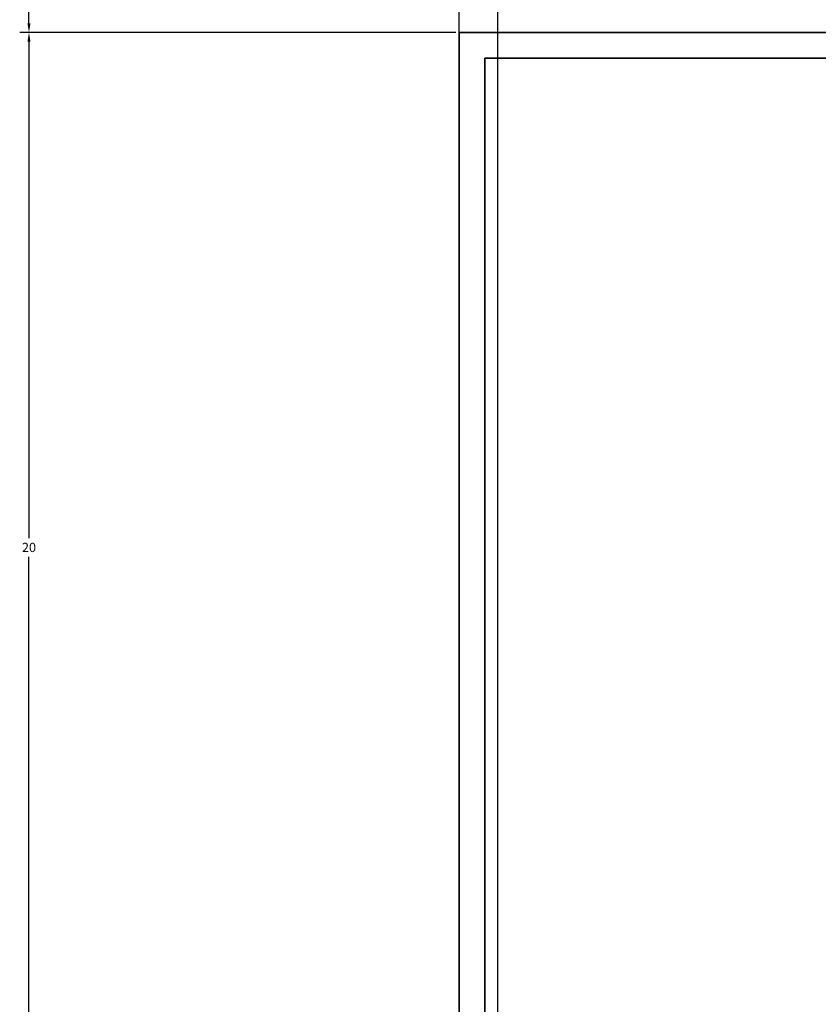
# Model space of a CAD drawing. Units: millimetres. Extents: x 446512 to 447461, y 70395 to 70610.
# Tile 2 of 39: x 446678.04 to 446693.54, y 70434.51 to 70453.63. Entities that reach past the tile are written whole.
import ezdxf

# ---------------------------------------------------------------- set-up
doc = ezdxf.new("R2010")
doc.units = ezdxf.units.MM
for name, color, linetype, lineweight in [('A-ANNO-DIMS', 2, 'Continuous', 18), ('A-CONS', 9, 'Continuous', 13), ('A-FURN', 7, 'Continuous', 35)]:
    doc.layers.add(name, color=color, linetype=linetype, lineweight=lineweight)
doc.styles.get("Standard").update_dxf_attribs({"font": 'arial.ttf'})
doc.dimstyles.get("Standard").update_dxf_attribs({"dimtxt": 0.18, "dimasz": 0.18, "dimexe": 0.18, "dimexo": 0.0625, "dimgap": 0.09, "dimtad": 0, "dimtih": 1, "dimtoh": 1, "dimdec": 4, "dimzin": 0, "dimdsep": 46, "dimtxsty": 'Standard', "dimcen": 0.09, "dimadec": 0, "dimazin": 0, "dimtfac": 1, "dimtdec": 4, "dimtofl": 0, "dimtmove": 0, "dimatfit": 3, "dimfxl": 1, "dimtolj": 1, "dimtzin": 0, "dimarcsym": 0})

# ---------------------------------------------------------------- blocks, each defined once
blk = doc.blocks.new('*D19')
at = {"layer": 'A-ANNO-DIMS', "color": 0, "lineweight": -2, "transparency": 16777216}
for p, q in [((446686.51, 70453.382), (446678.043, 70453.382)), ((446678.223, 70453.202), (446678.223, 70443.563)), ((446678.223, 70433.562), (446678.223, 70443.2)), ((446686.51, 70433.382), (446678.043, 70433.382))]:
    blk.add_line(p, q, dxfattribs=at)
at = {"layer": 'A-ANNO-DIMS', "color": 0, "transparency": 16777216}
for points in [[(446678.193, 70453.202), (446678.253, 70453.202), (446678.223, 70453.382)], [(446678.193, 70433.562), (446678.253, 70433.562), (446678.223, 70433.382)]]:
    blk.add_solid(points, dxfattribs=at)
at = {"layer": 'Defpoints', "color": 0, "transparency": 16777216}
for p in [(446678.223, 70453.382), (446686.573, 70453.382), (446686.573, 70433.382)]:
    blk.add_point(p, dxfattribs=at)
at = {"layer": 'A-ANNO-DIMS', "color": 0, "transparency": 16777216, "insert": (446678.223, 70443.382), "char_height": 0.18, "attachment_point": 5}
blk.add_mtext('\\A1;20', dxfattribs=at)
blk = doc.blocks.new('*D20')
at = {"layer": 'A-ANNO-DIMS', "color": 0, "lineweight": -2, "transparency": 16777216}
for p, q in [((446686.51, 70473.382), (446678.043, 70473.382)), ((446678.223, 70473.202), (446678.223, 70463.563)), ((446678.223, 70453.562), (446678.223, 70463.2)), ((446686.51, 70453.382), (446678.043, 70453.382))]:
    blk.add_line(p, q, dxfattribs=at)
at = {"layer": 'A-ANNO-DIMS', "color": 0, "transparency": 16777216}
for points in [[(446678.193, 70473.202), (446678.253, 70473.202), (446678.223, 70473.382)], [(446678.193, 70453.562), (446678.253, 70453.562), (446678.223, 70453.382)]]:
    blk.add_solid(points, dxfattribs=at)
at = {"layer": 'Defpoints', "color": 0, "transparency": 16777216}
for p in [(446678.223, 70473.382), (446686.573, 70473.382), (446686.573, 70453.382)]:
    blk.add_point(p, dxfattribs=at)
at = {"layer": 'A-ANNO-DIMS', "color": 0, "transparency": 16777216, "insert": (446678.223, 70463.382), "char_height": 0.18, "attachment_point": 5}
blk.add_mtext('\\A1;20', dxfattribs=at)
blk = doc.blocks.new('*D37')
at = {"layer": 'A-ANNO-DIMS', "color": 0, "lineweight": -2, "transparency": 16777216}
for p, q in [((446686.572846, 70433.44405), (446686.572846, 70578.17492)), ((446687.323552, 70428.838404), (446687.323552, 70578.17492)), ((446686.392846, 70577.99492), (446686.212846, 70577.99492)), ((446687.503552, 70577.99492), (446687.683552, 70577.99492))]:
    blk.add_line(p, q, dxfattribs=at)
at = {"layer": 'A-ANNO-DIMS', "color": 0, "transparency": 16777216}
for points in [[(446686.392846, 70578.02492), (446686.392846, 70577.96492), (446686.572846, 70577.99492)], [(446687.503552, 70578.02492), (446687.503552, 70577.96492), (446687.323552, 70577.99492)]]:
    blk.add_solid(points, dxfattribs=at)
at = {"layer": 'Defpoints', "color": 0, "transparency": 16777216}
for p in [(446687.323552, 70577.99492), (446686.572846, 70433.38155), (446687.323552, 70428.775904)]:
    blk.add_point(p, dxfattribs=at)
at = {"layer": 'A-ANNO-DIMS', "color": 0, "transparency": 16777216, "insert": (446686.948199, 70577.99492), "char_height": 0.18, "attachment_point": 5}
blk.add_mtext('\\A1;0.75', dxfattribs=at)
blk = doc.blocks.new('*D38')
at = {"layer": 'A-ANNO-DIMS', "color": 0, "lineweight": -2, "transparency": 16777216}
for p, q in [((446687.323552, 70428.838404), (446687.323552, 70578.17492)), ((446697.765686, 70428.838404), (446697.765686, 70578.17492)), ((446687.503552, 70577.99492), (446692.090383, 70577.99492)), ((446697.585686, 70577.99492), (446692.998855, 70577.99492))]:
    blk.add_line(p, q, dxfattribs=at)
at = {"layer": 'A-ANNO-DIMS', "color": 0, "transparency": 16777216}
for points in [[(446687.503552, 70578.02492), (446687.503552, 70577.96492), (446687.323552, 70577.99492)], [(446697.585686, 70578.02492), (446697.585686, 70577.96492), (446697.765686, 70577.99492)]]:
    blk.add_solid(points, dxfattribs=at)
at = {"layer": 'Defpoints', "color": 0, "transparency": 16777216}
for p in [(446697.765686, 70577.99492), (446687.323552, 70428.775904), (446697.765686, 70428.775904)]:
    blk.add_point(p, dxfattribs=at)
at = {"layer": 'A-ANNO-DIMS', "color": 0, "transparency": 16777216, "insert": (446692.544619, 70577.99492), "char_height": 0.18, "attachment_point": 5}
blk.add_mtext('\\A1;10.442', dxfattribs=at)

msp = doc.modelspace()

# ---------------------------------------------------------------- linework, layer by layer
at = {"layer": 'A-CONS'}
msp.add_point((446686.5728, 70453.3815), dxfattribs=at)
at = {"layer": 'A-FURN'}
for p, q in [((446686.5728, 70433.3815), (446686.5728, 70453.3815)), ((446686.5728, 70453.3815), (446746.5728, 70453.3815))]:
    msp.add_line(p, q, dxfattribs=at)
for points in [[(446686.5728, 70453.3815), (446729.0084, 70453.3815), (446729.0084, 70433.3815), (446686.5728, 70433.3815)], [(446687.0728, 70452.8815), (446728.5084, 70452.8815), (446728.5084, 70433.8815), (446687.0728, 70433.8815)]]:
    msp.add_lwpolyline(points, close=True, dxfattribs=at)

# ---------------------------------------------------------------- dimensions: what is measured, and where the dimension line sits
at = {"layer": 'A-ANNO-DIMS'}
for base, p1, p2, override, picture, middle in [((446687.3236, 70577.9949), (446686.5728, 70433.3815), (446687.3236, 70428.7759), {"dimdec": 2, "dimlfac": 1, "dimrnd": 0, "dimzin": 0, "dimdsep": 46, "dimlunit": 2}, '*D37', (446686.9482, 70577.9949)), ((446697.7657, 70577.9949), (446687.3236, 70428.7759), (446697.7657, 70428.7759), {"dimdec": 3, "dimlfac": 1, "dimrnd": 0, "dimzin": 0, "dimdsep": 46, "dimlunit": 2}, '*D38', (446692.5446, 70577.9949))]:
    dim = msp.add_linear_dim(base=base, p1=p1, p2=p2, dimstyle='Standard', override=override, dxfattribs=at)
    dim.commit()
    dim.dimension.update_dxf_attribs({"geometry": picture, "text_midpoint": middle})
for base, p1, p2, picture, middle in [((446678.2228, 70473.3816), (446686.5728, 70453.3815), (446686.5728, 70473.3816), '*D20', (446678.2228, 70463.3815)), ((446678.2228, 70453.3815), (446686.5728, 70433.3815), (446686.5728, 70453.3815), '*D19', (446678.2228, 70443.3815))]:
    dim = msp.add_linear_dim(base=base, p1=p1, p2=p2, angle=90, dimstyle='Standard', override={"dimdec": 0, "dimlfac": 1, "dimrnd": 0, "dimzin": 0, "dimdsep": 46, "dimlunit": 2}, dxfattribs=at)
    dim.commit()
    dim.dimension.update_dxf_attribs({"geometry": picture, "text_midpoint": middle})

doc.saveas('drawing.dxf')
